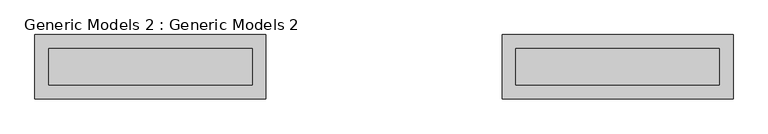
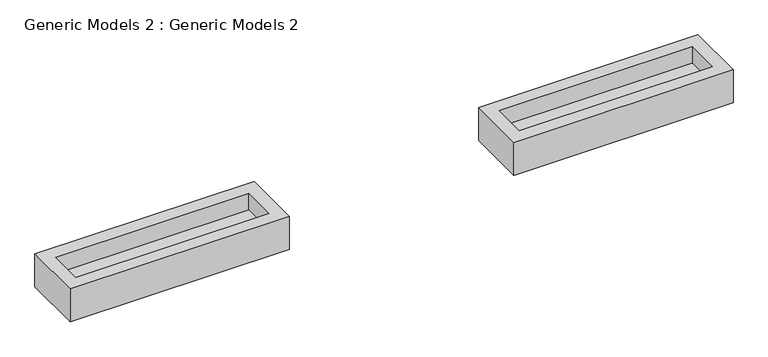
"""IFC4 building model written with IfcOpenShell, lengths in millimetres: proxy geometry, Generic Models 2 : Generic Models 2."""

from ifc_helpers import new_model, si_unit, origin, place, context, project, spatial, faceted_brep, source, transform, mapped, element, save


def generic_models_2_generic_models_2_98d2fe3e(model_context):
    return source(origin(), model_context, "Body", "Brep", [
        faceted_brep([(-16338.7991683, -4185.4496381, 4114.8), (-20170.2183666, -4185.4496381, 4114.8), (-20170.2183666, -5252.2496381, 4114.8), (-16338.7991683, -5252.2496381, 4114.8), (-16567.3991683, -4414.0496381, 4114.8), (-16567.3991683, -5023.6496381, 4114.8), (-19941.6183666, -5023.6496381, 4114.8), (-19941.6183666, -4414.0496381, 4114.8), (-16338.7991683, -4185.4496381, 3505.2), (-16338.7991683, -5252.2496381, 3505.2), (-20170.2183666, -5252.2496381, 3505.2), (-20170.2183666, -4185.4496381, 3505.2), (-16567.3991683, -4414.0496381, 3810.0), (-19941.6183666, -4414.0496381, 3810.0), (-19941.6183666, -5023.6496381, 3810.0), (-16567.3991683, -5023.6496381, 3810.0)], [[[0, 1, 2, 3], [4, 5, 6, 7]], [[8, 9, 10, 11]], [[1, 0, 8, 11]], [[2, 1, 11, 10]], [[3, 2, 10, 9]], [[0, 3, 9, 8]], [[12, 13, 14, 15]], [[12, 15, 5, 4]], [[15, 14, 6, 5]], [[14, 13, 7, 6]], [[13, 12, 4, 7]]]),
        faceted_brep([(-8587.8183666, -4185.4496381, 4114.8), (-12419.237565, -4185.4496381, 4114.8), (-12419.237565, -5252.2496381, 4114.8), (-8587.8183666, -5252.2496381, 4114.8), (-8816.4183666, -4414.0496381, 4114.8), (-8816.4183666, -5023.6496381, 4114.8), (-12190.637565, -5023.6496381, 4114.8), (-12190.637565, -4414.0496381, 4114.8), (-8587.8183666, -4185.4496381, 3505.2), (-8587.8183666, -5252.2496381, 3505.2), (-12419.237565, -5252.2496381, 3505.2), (-12419.237565, -4185.4496381, 3505.2), (-8816.4183666, -4414.0496381, 3810.0), (-12190.637565, -4414.0496381, 3810.0), (-12190.637565, -5023.6496381, 3810.0), (-8816.4183666, -5023.6496381, 3810.0)], [[[0, 1, 2, 3], [4, 5, 6, 7]], [[8, 9, 10, 11]], [[1, 0, 8, 11]], [[2, 1, 11, 10]], [[3, 2, 10, 9]], [[0, 3, 9, 8]], [[12, 13, 14, 15]], [[12, 15, 5, 4]], [[15, 14, 6, 5]], [[14, 13, 7, 6]], [[13, 12, 4, 7]]]),
    ])


if __name__ == "__main__":
    model = new_model("IFC4")
    model_context = context("Model", 3, world=origin())
    ifc_project = project(units=[si_unit("LENGTHUNIT", "METRE", prefix="MILLI")], contexts=[model_context])
    site = spatial("IfcSite", under=ifc_project)
    building = spatial("IfcBuilding", under=site)
    placement = place(None, origin())
    generic_models_2_generic_models_2_shape = generic_models_2_generic_models_2_98d2fe3e(model_context)
    element("IfcBuildingElementProxy", 1, Name="Generic Models 2 : Generic Models 2", ObjectType="Generic Models 2 : Generic Models 2", at=placement, inside=building, context=model_context, shape_type="MappedRepresentation", body=[
        mapped(generic_models_2_generic_models_2_shape, transform((0.0, 0.0, 0.0), x_axis=(1.0, 0.0, 0.0), y_axis=(0.0, 1.0, 0.0), z_axis=(0.0, 0.0, 1.0))),
    ])
    save(model, "model.ifc")
